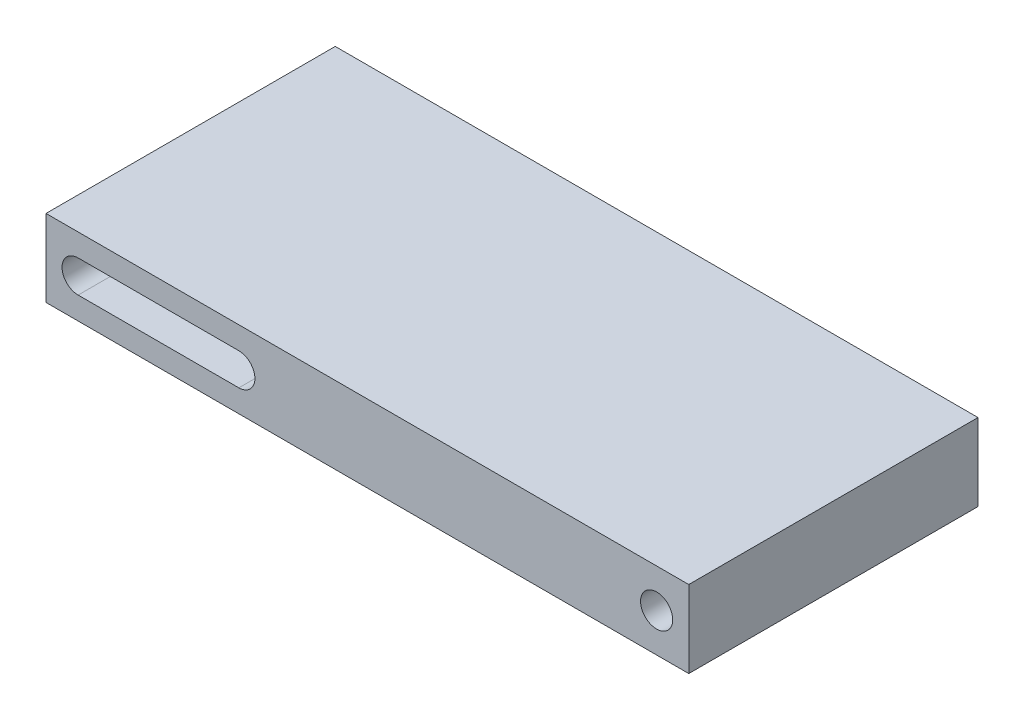
from build123d import *

# Parameters (mm, degrees)
PLATE_PROFILE_SKETCH_W          = 100
PLATE_PROFILE_SKETCH_H          = 12
BASE_PLATE_100X12X45_DEPTH      = 22.5
THROUGH_SLOT_AND_HOLE_CUT_REACH = 69.535
SLOT_AND_HOLE_SKETCH_R          = 2.5


with BuildPart() as part:
    # Plate Profile Sketch → Base Plate 100x12x45 (new, symmetric)
    with BuildSketch(Plane.XY):
        Rectangle(PLATE_PROFILE_SKETCH_W, PLATE_PROFILE_SKETCH_H)
    extrude(amount=BASE_PLATE_100X12X45_DEPTH, both=True)

    # Slot and Hole Sketch → Through Slot and Hole Cut (cut, up to next)
    with BuildSketch(Plane.XY.offset(22.5), mode=Mode.PRIVATE) as through_slot_and_hole_cut_sk1:
        with Locations((45, 0)):
            Circle(SLOT_AND_HOLE_SKETCH_R)
    through_slot_and_hole_cut_tool1 = extrude(through_slot_and_hole_cut_sk1.sketch, amount=-THROUGH_SLOT_AND_HOLE_CUT_REACH, mode=Mode.PRIVATE) & part.part
    # Slot and Hole Sketch → Through Slot and Hole Cut (cut, up to next)
    with BuildSketch(Plane.XY.offset(22.5), mode=Mode.PRIVATE) as through_slot_and_hole_cut_sk2:
        with BuildLine():
            Line((-45, 2.5), (-20, 2.5))
            ThreePointArc((-20, 2.5), (-17.5, 0), (-20, -2.5))
            Line((-20, -2.5), (-45, -2.5))
            ThreePointArc((-45, -2.5), (-47.5, 0), (-45, 2.5))
        make_face()
    through_slot_and_hole_cut_tool2 = extrude(through_slot_and_hole_cut_sk2.sketch, amount=-THROUGH_SLOT_AND_HOLE_CUT_REACH, mode=Mode.PRIVATE) & part.part
    add(through_slot_and_hole_cut_tool1.solids().sort_by_distance((45, 0, 22.5))[0], mode=Mode.SUBTRACT)
    add(through_slot_and_hole_cut_tool2.solids().sort_by_distance((-32.5, 0, 22.5))[0], mode=Mode.SUBTRACT)


solid = part.part
